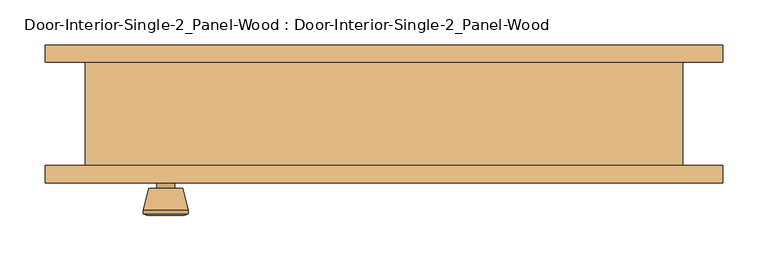
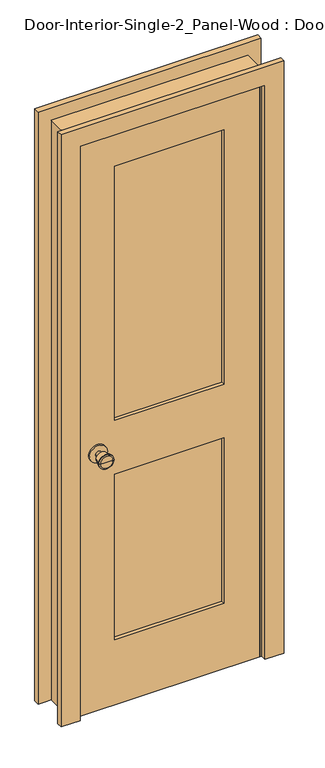
"""IFC4 building model written with IfcOpenShell, lengths in millimetres: door geometry, Door-Interior-Single-2_Panel-Wood : Door-Interior-Single-2_Panel-Wood."""

from ifc_helpers import new_model, si_unit, point, frame, frame_2d, origin, place, context, project, spatial, polyline, circle_curve, trimmed, segment, composite_curve, outline, extrude, faceted_brep, source, transform, mapped, element, save
from ifc_brep_helpers import plane_surface, cylinder_surface, revolved_surface, advanced_brep


def door_interior_single_2_panel_wood_door_interior_single_2_03d66c98(model_context):
    return source(origin(), model_context, "Body", "SolidModel", [
        advanced_brep(
        [(-241.3, -13.05, 914.4), (-251.3, -13.05, 914.4), (-231.3, -13.05, 914.4), (-220.8241324, 35.95, 914.4), (-261.7758676, 35.95, 914.4), (-241.3, 35.95, 914.4), (-216.3, 34.1221319, 914.4), (-266.3, 34.1221319, 914.4), (-216.3, 30.6584537, 914.4), (-266.3, 30.6584537, 914.4), (-222.663764, 5.95, 914.4), (-259.936236, 5.95, 914.4), (-231.3, 5.95, 914.4), (-251.3, 5.95, 914.4)],
        [
            (0, 1),
            (1, 2, circle_curve(frame((-241.3, -13.05, 914.4), z_axis=(0.0, -1.0, 0.0), x_axis=(-1.0, 0.0, 0.0)), 10.0)),
            (2, 0),
            (2, 1, circle_curve(frame((-241.3, -13.05, 914.4), z_axis=(0.0, -1.0, 0.0), x_axis=(-1.0, 0.0, 0.0)), 10.0)),
            (3, 4, circle_curve(frame((-241.3, 35.95, 914.4), z_axis=(0.0, 1.0, 0.0), x_axis=(-1.0, 0.0, 0.0)), 20.4758676)),
            (4, 5),
            (5, 3),
            (4, 3, circle_curve(frame((-241.3, 35.95, 914.4), z_axis=(0.0, 1.0, 0.0), x_axis=(-1.0, 0.0, 0.0)), 20.4758676)),
            (6, 7, circle_curve(frame((-241.3, 34.1221319, 914.4), z_axis=(0.0, 1.0, 0.0), x_axis=(-1.0, 0.0, 0.0)), 25.0)),
            (7, 4),
            (3, 6),
            (7, 6, circle_curve(frame((-241.3, 34.1221319, 914.4), z_axis=(0.0, 1.0, 0.0), x_axis=(-1.0, 0.0, 0.0)), 25.0)),
            (8, 9, circle_curve(frame((-241.3, 30.6584537, 914.4), z_axis=(0.0, 1.0, 0.0), x_axis=(-1.0, 0.0, 0.0)), 25.0)),
            (9, 7),
            (6, 8),
            (9, 8, circle_curve(frame((-241.3, 30.6584537, 914.4), z_axis=(0.0, 1.0, 0.0), x_axis=(-1.0, 0.0, 0.0)), 25.0)),
            (10, 11, circle_curve(frame((-241.3, 5.95, 914.4), z_axis=(0.0, 1.0, 0.0), x_axis=(-1.0, 0.0, 0.0)), 18.636236)),
            (11, 9),
            (8, 10),
            (11, 10, circle_curve(frame((-241.3, 5.95, 914.4), z_axis=(0.0, 1.0, 0.0), x_axis=(-1.0, 0.0, 0.0)), 18.636236)),
            (12, 13, circle_curve(frame((-241.3, 5.95, 914.4), z_axis=(0.0, 1.0, 0.0), x_axis=(-1.0, 0.0, 0.0)), 10.0)),
            (13, 11),
            (10, 12),
            (13, 12, circle_curve(frame((-241.3, 5.95, 914.4), z_axis=(0.0, 1.0, 0.0), x_axis=(-1.0, 0.0, 0.0)), 10.0)),
            (1, 13),
            (12, 2),
        ],
        [
            plane_surface(frame((-241.3, -13.05, 914.4), z_axis=(0.0, -1.0, 0.0), x_axis=(-1.0, 0.0, 0.0))),
            plane_surface(frame((-241.3, 35.95, 914.4), z_axis=(0.0, 1.0, 0.0), x_axis=(-1.0, 0.0, 0.0))),
            revolved_surface(polyline([(-261.7758676, 35.95, 914.4), (-266.3, 34.1221319, 914.4)]), (-241.3, -13.05, 914.4), (0.0, -1.0, 0.0)),
            cylinder_surface(frame((-241.3, -13.05, 914.4), z_axis=(0.0, -1.0, 0.0), x_axis=(-1.0, 0.0, 0.0)), 25.0),
            revolved_surface(polyline([(-266.3, 30.6584537, 914.4), (-259.936236, 5.95, 914.4)]), (-241.3, -13.05, 914.4), (0.0, -1.0, 0.0)),
            plane_surface(frame((-241.3, 5.95, 914.4), z_axis=(0.0, -1.0, 0.0), x_axis=(-1.0, 0.0, 0.0))),
            cylinder_surface(frame((-241.3, -13.05, 914.4), z_axis=(0.0, -1.0, 0.0), x_axis=(-1.0, 0.0, 0.0)), 10.0),
        ],
        [
            (0, [[1, 2, 3]]),
            (0, [[-3, 4, -1]]),
            (1, [[5, 6, 7]]),
            (1, [[8, -7, -6]]),
            (2, [[9, 10, -5, 11]]),
            (2, [[12, -11, -8, -10]]),
            (3, [[13, 14, -9, 15]]),
            (3, [[16, -15, -12, -14]]),
            (4, [[17, 18, -13, 19]]),
            (4, [[20, -19, -16, -18]]),
            (5, [[21, 22, -17, 23]]),
            (5, [[24, -23, -20, -22]]),
            (6, [[-2, 25, -21, 26]]),
            (6, [[-4, -26, -24, -25]]),
        ],
    ),
        extrude(outline(composite_curve([segment(trimmed(circle_curve(frame_2d((914.4, -241.3)), 30.0), [point((914.4, -271.3))], [point((914.4, -211.3))], False, "CARTESIAN"), True, "CONTINUOUS"), segment(trimmed(circle_curve(frame_2d((914.4, -241.3)), 30.0), [point((914.4, -211.3))], [point((914.4, -271.3))], False, "CARTESIAN"), True, "CONTINUOUS")], self_intersect=False)), frame((0.0, -19.05, 0.0), z_axis=(0.0, 1.0, 0.0), x_axis=(0.0, 0.0, 1.0)), (0.0, 0.0, 1.0), 6.0),
        advanced_brep(
        [(-241.3, -59.975, 914.4), (-231.3, -59.975, 914.4), (-251.3, -59.975, 914.4), (-220.8241324, -108.975, 914.4), (-241.3, -108.975, 914.4), (-261.7758676, -108.975, 914.4), (-216.3, -107.1471319, 914.4), (-266.3, -107.1471319, 914.4), (-216.3, -103.6834537, 914.4), (-266.3, -103.6834537, 914.4), (-222.663764, -78.975, 914.4), (-259.936236, -78.975, 914.4), (-231.3, -78.975, 914.4), (-251.3, -78.975, 914.4)],
        [
            (0, 1),
            (1, 2, circle_curve(frame((-241.3, -59.975, 914.4), z_axis=(0.0, 1.0, 0.0), x_axis=(-1.0, 0.0, 0.0)), 10.0)),
            (2, 0),
            (2, 1, circle_curve(frame((-241.3, -59.975, 914.4), z_axis=(0.0, 1.0, 0.0), x_axis=(-1.0, 0.0, 0.0)), 10.0)),
            (3, 4),
            (4, 5),
            (5, 3, circle_curve(frame((-241.3, -108.975, 914.4), z_axis=(0.0, -1.0, 0.0), x_axis=(-1.0, 0.0, 0.0)), 20.4758676)),
            (3, 5, circle_curve(frame((-241.3, -108.975, 914.4), z_axis=(0.0, -1.0, 0.0), x_axis=(-1.0, 0.0, 0.0)), 20.4758676)),
            (6, 3),
            (5, 7),
            (7, 6, circle_curve(frame((-241.3, -107.1471319, 914.4), z_axis=(0.0, -1.0, 0.0), x_axis=(-1.0, 0.0, 0.0)), 25.0)),
            (6, 7, circle_curve(frame((-241.3, -107.1471319, 914.4), z_axis=(0.0, -1.0, 0.0), x_axis=(-1.0, 0.0, 0.0)), 25.0)),
            (8, 6),
            (7, 9),
            (9, 8, circle_curve(frame((-241.3, -103.6834537, 914.4), z_axis=(0.0, -1.0, 0.0), x_axis=(-1.0, 0.0, 0.0)), 25.0)),
            (8, 9, circle_curve(frame((-241.3, -103.6834537, 914.4), z_axis=(0.0, -1.0, 0.0), x_axis=(-1.0, 0.0, 0.0)), 25.0)),
            (10, 8),
            (9, 11),
            (11, 10, circle_curve(frame((-241.3, -78.975, 914.4), z_axis=(0.0, -1.0, 0.0), x_axis=(-1.0, 0.0, 0.0)), 18.636236)),
            (10, 11, circle_curve(frame((-241.3, -78.975, 914.4), z_axis=(0.0, -1.0, 0.0), x_axis=(-1.0, 0.0, 0.0)), 18.636236)),
            (12, 10),
            (11, 13),
            (13, 12, circle_curve(frame((-241.3, -78.975, 914.4), z_axis=(0.0, -1.0, 0.0), x_axis=(-1.0, 0.0, 0.0)), 10.0)),
            (12, 13, circle_curve(frame((-241.3, -78.975, 914.4), z_axis=(0.0, -1.0, 0.0), x_axis=(-1.0, 0.0, 0.0)), 10.0)),
            (1, 12),
            (13, 2),
        ],
        [
            plane_surface(frame((-241.3, -59.975, 914.4), z_axis=(0.0, 1.0, 0.0), x_axis=(-1.0, 0.0, 0.0))),
            plane_surface(frame((-241.3, -108.975, 914.4), z_axis=(0.0, -1.0, 0.0), x_axis=(-1.0, 0.0, 0.0))),
            revolved_surface(polyline([(-261.7758676, -108.975, 914.4), (-266.3, -107.1471319, 914.4)]), (-241.3, -59.975, 914.4), (0.0, 1.0, 0.0)),
            cylinder_surface(frame((-241.3, -59.975, 914.4), z_axis=(0.0, 1.0, 0.0), x_axis=(-1.0, 0.0, 0.0)), 25.0),
            revolved_surface(polyline([(-266.3, -103.6834537, 914.4), (-259.936236, -78.975, 914.4)]), (-241.3, -59.975, 914.4), (0.0, 1.0, 0.0)),
            plane_surface(frame((-241.3, -78.975, 914.4), z_axis=(0.0, 1.0, 0.0), x_axis=(-1.0, 0.0, 0.0))),
            cylinder_surface(frame((-241.3, -59.975, 914.4), z_axis=(0.0, 1.0, 0.0), x_axis=(-1.0, 0.0, 0.0)), 10.0),
        ],
        [
            (0, [[1, 2, 3]]),
            (0, [[-3, 4, -1]]),
            (1, [[5, 6, 7]]),
            (1, [[-6, -5, 8]]),
            (2, [[9, -7, 10, 11]]),
            (2, [[-10, -8, -9, 12]]),
            (3, [[13, -11, 14, 15]]),
            (3, [[-14, -12, -13, 16]]),
            (4, [[17, -15, 18, 19]]),
            (4, [[-18, -16, -17, 20]]),
            (5, [[21, -19, 22, 23]]),
            (5, [[-22, -20, -21, 24]]),
            (6, [[25, -23, 26, -2]]),
            (6, [[-26, -24, -25, -4]]),
        ],
    ),
        extrude(outline(composite_curve([segment(trimmed(circle_curve(frame_2d((914.4, -241.3)), 30.0), [point((914.4, -271.3))], [point((914.4, -211.3))], False, "CARTESIAN"), True, "CONTINUOUS"), segment(trimmed(circle_curve(frame_2d((914.4, -241.3)), 30.0), [point((914.4, -211.3))], [point((914.4, -271.3))], False, "CARTESIAN"), True, "CONTINUOUS")], self_intersect=False)), frame((0.0, -59.975, 0.0), z_axis=(0.0, 1.0, 0.0), x_axis=(0.0, 0.0, 1.0)), (0.0, 0.0, 1.0), 6.0),
        faceted_brep([(330.2, -53.975, 0.0), (304.8, -53.975, 0.0), (304.8, -19.05, 0.0), (292.1, -19.05, 0.0), (292.1, 15.875, 0.0), (304.8, 15.875, 0.0), (304.8, 60.325, 0.0), (330.2, 60.325, 0.0), (330.2, 60.325, 2057.4), (330.2, -53.975, 2057.4), (304.8, 60.325, 2032.0), (-304.8, 60.325, 2032.0), (-304.8, 60.325, 0.0), (-330.2, 60.325, 0.0), (-330.2, 60.325, 2057.4), (304.8, 15.875, 2032.0), (292.1, 15.875, 2019.3), (-292.1, 15.875, 2019.3), (-292.1, 15.875, 0.0), (-304.8, 15.875, 0.0), (-304.8, 15.875, 2032.0), (292.1, -19.05, 2019.3), (304.8, -19.05, 2032.0), (-304.8, -19.05, 2032.0), (-304.8, -19.05, 0.0), (-292.1, -19.05, 0.0), (-292.1, -19.05, 2019.3), (304.8, -53.975, 2032.0), (-330.2, -53.975, 2057.4), (-330.2, -53.975, 0.0), (-304.8, -53.975, 0.0), (-304.8, -53.975, 2032.0)], [[[0, 1, 2, 3, 4, 5, 6, 7]], [[7, 8, 9, 0]], [[6, 10, 11, 12, 13, 14, 8, 7]], [[5, 15, 10, 6]], [[4, 16, 17, 18, 19, 20, 15, 5]], [[3, 21, 16, 4]], [[2, 22, 23, 24, 25, 26, 21, 3]], [[1, 27, 22, 2]], [[0, 9, 28, 29, 30, 31, 27, 1]], [[8, 14, 28, 9]], [[15, 20, 11, 10]], [[21, 26, 17, 16]], [[27, 31, 23, 22]], [[29, 13, 12, 19, 18, 25, 24, 30]], [[14, 13, 29, 28]], [[20, 19, 12, 11]], [[26, 25, 18, 17]], [[31, 30, 24, 23]]]),
        extrude(outline(polyline([(2032.0, -304.8), (0.0, -304.8), (0.0, 304.8), (2032.0, 304.8), (2032.0, -304.8)]), holes=[polyline([(1912.9375, -184.15), (1912.9375, 184.15), (1009.65, 184.15), (1009.65, -184.15), (1912.9375, -184.15)]), polyline([(819.15, -184.15), (819.15, 184.15), (231.775, 184.15), (231.775, -184.15), (819.15, -184.15)])]), frame((0.0, -53.975, 0.0), z_axis=(0.0, 1.0, 0.0), x_axis=(0.0, 0.0, 1.0)), (0.0, 0.0, 1.0), 34.925),
        extrude(outline(polyline([(184.15, -30.6916667), (184.15, -42.3333333), (-184.15, -42.3333333), (-184.15, -30.6916667), (184.15, -30.6916667)])), frame((0.0, 0.0, 1009.65), z_axis=(0.0, 0.0, 1.0), x_axis=(1.0, 0.0, 0.0)), (0.0, 0.0, 1.0), 903.2875),
        extrude(outline(polyline([(184.15, -30.6916667), (184.15, -42.3333333), (-184.15, -42.3333333), (-184.15, -30.6916667), (184.15, -30.6916667)])), frame((0.0, 0.0, 231.775), z_axis=(0.0, 0.0, 1.0), x_axis=(1.0, 0.0, 0.0)), (0.0, 0.0, 1.0), 587.375),
        extrude(outline(polyline([(0.0, 374.65), (2101.85, 374.65), (2101.85, -374.65), (0.0, -374.65), (0.0, -311.15), (2038.35, -311.15), (2038.35, 311.15), (0.0, 311.15), (0.0, 374.65)])), frame((0.0, -73.025, 0.0), z_axis=(0.0, 1.0, 0.0), x_axis=(0.0, 0.0, 1.0)), (0.0, 0.0, 1.0), 19.05),
        extrude(outline(polyline([(0.0, 374.65), (2101.85, 374.65), (2101.85, -374.65), (0.0, -374.65), (0.0, -311.15), (2038.35, -311.15), (2038.35, 311.15), (0.0, 311.15), (0.0, 374.65)])), frame((0.0, 60.325, 0.0), z_axis=(0.0, 1.0, 0.0), x_axis=(0.0, 0.0, 1.0)), (0.0, 0.0, 1.0), 19.05),
    ])


if __name__ == "__main__":
    model = new_model("IFC4")
    model_context = context("Model", 3, world=origin())
    ifc_project = project(units=[si_unit("LENGTHUNIT", "METRE", prefix="MILLI")], contexts=[model_context])
    site = spatial("IfcSite", under=ifc_project)
    building = spatial("IfcBuilding", under=site)
    placement = place(None, origin())
    door_interior_single_2_panel_wood_door_interior_single_2_shape = door_interior_single_2_panel_wood_door_interior_single_2_03d66c98(model_context)
    element("IfcDoor", 1, ObjectType="Door-Interior-Single-2_Panel-Wood : Door-Interior-Single-2_Panel-Wood", at=placement, inside=building, context=model_context, shape_type="MappedRepresentation", body=[
        mapped(door_interior_single_2_panel_wood_door_interior_single_2_shape, transform((0.0, 0.0, 0.0), x_axis=(1.0, 0.0, 0.0), y_axis=(0.0, 1.0, 0.0), z_axis=(0.0, 0.0, 1.0))),
    ])
    save(model, "model.ifc")

# Revit data of these elements
# Type "Door-Interior-Single-2_Panel-Wood : Door-Interior-Single-2_Panel-Wood"
#   Type Mark = "12"
#   Assembly Code = "C1020300"
#   Analytic Construction = "Wooden"
#   Top Rail = 0' - 4 11/16"
#   Thickness = 0' - 1 3/8"
#   Thermal Resistance (R) = 2.5876 (h·ft²·°F)/BTU
#   Swing Angle [instance default] = 90.00°
#   Stiles = 0' - 4 3/4"
#   Rough Width = 2' - 2"
#   Rough Height = 6' - 9"
#   Lock Rail = 0' - 7 1/2"
#   Height = 6' - 8"
#   Width = 2' - 0"
#   Heat Transfer Coefficient (U) = 0.3865 BTU/(h·ft²·°F)
#   Bottom Rail = 0' - 9 1/8"
#   Trim Material = Cherry
#   Panel Material = Cherry
#   Frame Material = Cherry
#   Door Handle Material = Aluminum
#   Visual Light Transmittance = 0
#   Solar Heat Gain Coefficient = 0
#   Wall Closure = (empty or 0)
#   Function = (empty or 0)
# Element 1 (IfcDoor, "Door-Interior-Single-2_Panel-Wood : Door-Interior-Single-2_Panel-Wood")
#   Materials on its faces: "Cherry", "Aluminum"
# Materials
#   "Cherry": class "Wood", colour RGB 226 177 128, transparency 0, Description = "Prunus Serotina", Cost = 0
#   "Aluminum": class "Metal", colour RGB 247 247 247, transparency 0, Description = "Aluminum 6061", Cost = 0
